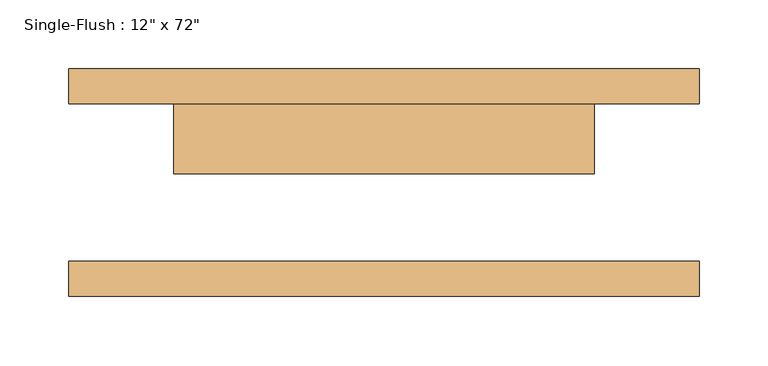
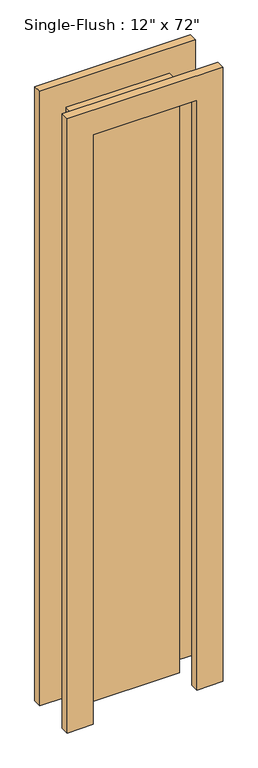
"""IFC4 building model written with IfcOpenShell, lengths in millimetres: door geometry."""

from ifc_helpers import new_model, si_unit, frame, origin, origin_with_axes, place, context, project, spatial, polyline, outline, extrude, source, transform, mapped, element, save


def door_b768bedd(model_context):
    return source(origin(), model_context, "Body", "SweptSolid", [
        extrude(outline(polyline([(1905.0, -228.6), (0.0, -228.6), (0.0, -152.4), (1828.8, -152.4), (1828.8, 152.4), (0.0, 152.4), (0.0, 228.6), (1905.0, 228.6), (1905.0, -228.6)])), frame((0.0, 57.15, 0.0), z_axis=(0.0, 1.0, 0.0), x_axis=(0.0, 0.0, 1.0)), (0.0, 0.0, 1.0), 25.4),
        extrude(outline(polyline([(1905.0, 228.6), (1905.0, -228.6), (0.0, -228.6), (0.0, -152.4), (1828.8, -152.4), (1828.8, 152.4), (0.0, 152.4), (0.0, 228.6), (1905.0, 228.6)])), frame((0.0, -82.55, 0.0), z_axis=(0.0, 1.0, 0.0), x_axis=(0.0, 0.0, 1.0)), (0.0, 0.0, 1.0), 25.4),
        extrude(outline(polyline([(152.4, 6.35), (-152.4, 6.35), (-152.4, 57.15), (152.4, 57.15), (152.4, 6.35)])), origin_with_axes(), (0.0, 0.0, 1.0), 1828.8),
    ])


if __name__ == "__main__":
    model = new_model("IFC4")
    model_context = context("Model", 3, world=origin())
    ifc_project = project(units=[si_unit("LENGTHUNIT", "METRE", prefix="MILLI")], contexts=[model_context])
    site = spatial("IfcSite", under=ifc_project)
    building = spatial("IfcBuilding", under=site)
    placement = place(None, origin())
    door_shape = door_b768bedd(model_context)
    element("IfcDoor", 1, ObjectType="Single-Flush : 12\" x 72\"", at=placement, inside=building, context=model_context, shape_type="MappedRepresentation", body=[
        mapped(door_shape, transform((0.0, 0.0, 0.0), x_axis=(1.0, 0.0, 0.0), y_axis=(0.0, 1.0, 0.0), z_axis=(0.0, 0.0, 1.0))),
    ])
    save(model, "model.ifc")

# Revit data of these elements
# Type "Single-Flush : 12\" x 72\""
#   Type Mark = "5"
#   Construction Type Id = "MDOOR"
#   Assembly Code = "C1020"
#   Analytic Construction = "Metal"
#   Thickness = 0' - 2"
#   Heat Transfer Coefficient (U) = 0.651978 BTU/(h·ft²·°F)
#   Height = 6' - 0"
#   Trim Projection Ext = 0' - 1"
#   Trim Projection Int = 0' - 1"
#   Trim Width = 0' - 3"
#   Width = 1' - 0"
#   Define Thermal Properties by = 1
#   Define Thermal Properties by = 1
#   Door Material = Door - Panel
#   Frame Material = Door - Frame
#   Visual Light Transmittance = 0
#   Solar Heat Gain Coefficient = 0
#   Function = (empty or 0)
#   Wall Closure = (empty or 0)
# Element 1 (IfcDoor, "Single-Flush : 12\" x 72\"")
#   Materials on its faces: "Door - Frame", "Door - Panel"
# Materials
#   "Door - Panel": class "Wood", colour RGB 210 159 95, transparency 0, Cost = 0
#   "Door - Frame": colour RGB 118 70 51, transparency 0, Cost = 0
